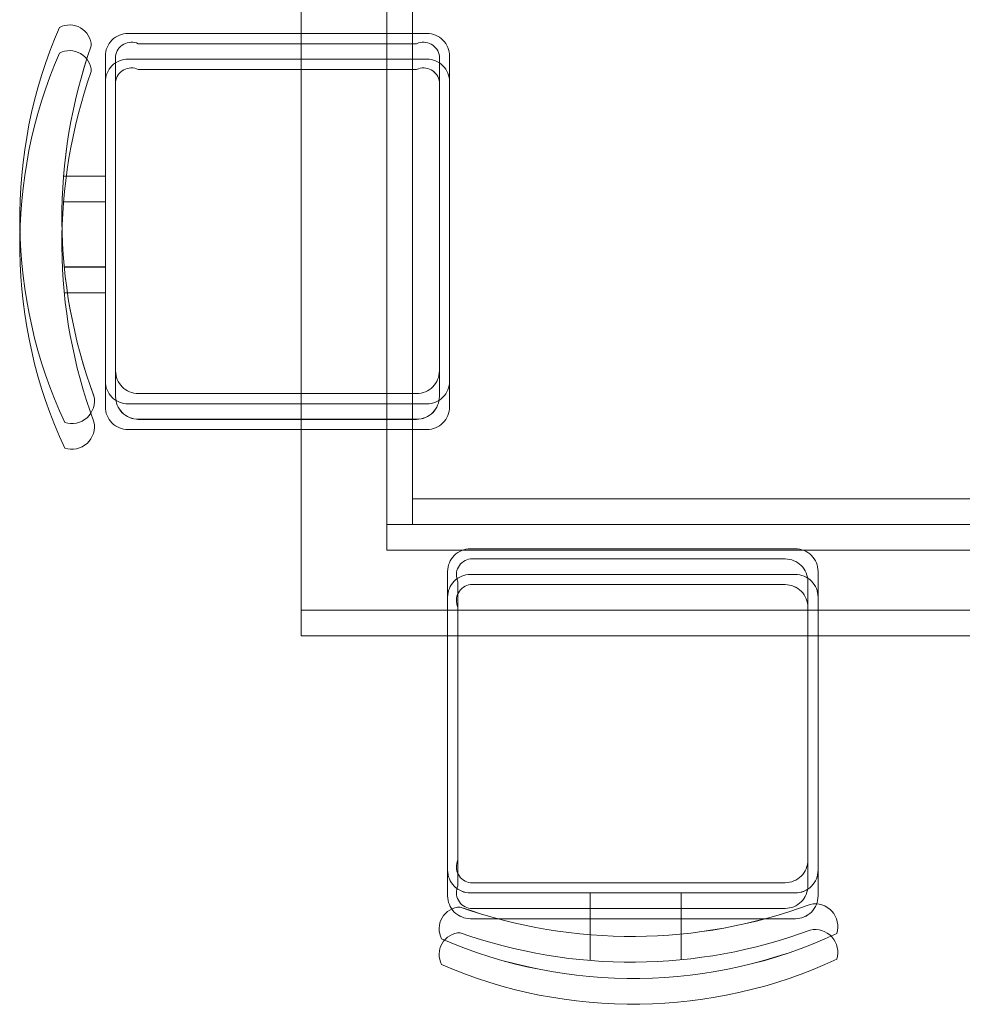
# Model space of a CAD drawing. Units: inches. Extents: x 1885 to 2748, y 783 to 2421.
# Tile 81 of 117: x 2129 to 2156, y 2066 to 2095. Entities that reach past the tile are written whole.
import ezdxf

# ---------------------------------------------------------------- set-up
doc = ezdxf.new("R2010")
doc.units = ezdxf.units.IN
doc.layers.add('A-FURN', color=8, linetype='Continuous', lineweight=13)

# ---------------------------------------------------------------- blocks, each defined once
blk = doc.blocks.new('TABLE-DINING-RECT')
for points in [[(-0.004, 23.421), (37.776, 23.421), (37.776, 0.754), (-0.004, 0.754)], [(-0.004, 23.421), (37.776, 23.421), (37.776, 0.753), (-0.004, 0.753)], [(-0.004, 22.666), (37.776, 22.666), (37.776, -0.002), (-0.004, -0.002)], [(-0.004, 22.665), (37.776, 22.665), (37.776, -0.002), (-0.004, -0.002)], [(2.515, 20.903), (35.257, 20.903), (35.257, 3.272), (2.515, 3.272)], [(2.515, 20.902), (35.257, 20.902), (35.257, 3.272), (2.515, 3.272)], [(2.515, 20.147), (35.257, 20.147), (35.257, 2.517), (2.515, 2.517)], [(2.515, 20.147), (35.257, 20.147), (35.257, 2.516), (2.515, 2.516)], [(3.27, 20.147), (34.501, 20.147), (34.501, 4.028), (3.27, 4.028)], [(3.27, 20.147), (34.501, 20.147), (34.501, 4.027), (3.27, 4.027)], [(3.27, 19.391), (34.501, 19.391), (34.501, 3.272), (3.27, 3.272)], [(3.27, 19.391), (34.501, 19.391), (34.501, 3.272), (3.27, 3.272)]]:
    blk.add_lwpolyline(points, close=True)

msp = doc.modelspace()

# ---------------------------------------------------------------- linework, layer by layer
at = {"layer": 'A-FURN'}
for points in [[(2130.918, 2084.243, -0.578392), (2130.06, 2083.463, -0.214524), (2129.905, 2095.078, -0.552014), (2130.84, 2094.533, 0.175809), (2130.918, 2084.243)], [(2130.918, 2084.242, -0.578392), (2130.06, 2083.463, -0.214524), (2129.905, 2095.078, -0.552014), (2130.84, 2094.532, 0.175809), (2130.918, 2084.242)], [(2131.253, 2094.232, -0.414214), (2131.921, 2094.901), (2140.705, 2094.901, -0.414214), (2141.373, 2094.232), (2141.373, 2084.679, -0.414214), (2140.705, 2084.011), (2131.921, 2084.011, -0.414214), (2131.253, 2084.679), (2131.253, 2094.232)], [(2131.253, 2094.232, -0.414214), (2131.921, 2094.9), (2140.705, 2094.9, -0.414214), (2141.373, 2094.232), (2141.373, 2084.679, -0.414214), (2140.705, 2084.011), (2131.921, 2084.011, -0.414214), (2131.253, 2084.679), (2131.253, 2094.232)], [(2130.918, 2083.487, -0.578392), (2130.06, 2082.708, -0.214524), (2129.905, 2094.323, -0.552014), (2130.84, 2093.777, 0.175809), (2130.918, 2083.487)], [(2130.918, 2083.487, -0.578392), (2130.06, 2082.707, -0.214524), (2129.905, 2094.323, -0.552014), (2130.84, 2093.777, 0.175809), (2130.918, 2083.487)], [(2131.253, 2093.477, -0.414214), (2131.921, 2094.145), (2140.705, 2094.145, -0.414214), (2141.373, 2093.477), (2141.373, 2083.924, -0.414214), (2140.705, 2083.255), (2131.921, 2083.255, -0.414214), (2131.253, 2083.924), (2131.253, 2093.477)], [(2131.253, 2093.476, -0.414214), (2131.921, 2094.145), (2140.705, 2094.145, -0.414214), (2141.373, 2093.476), (2141.373, 2083.923, -0.414214), (2140.705, 2083.255), (2131.921, 2083.255, -0.414214), (2131.253, 2083.923), (2131.253, 2093.476)], [(2131.253, 2088.035), (2130.045, 2088.035, 0.064759)], [(2131.253, 2088.034), (2130.045, 2088.034, 0.064759)], [(2131.253, 2087.279), (2130.045, 2087.279, 0.064759)], [(2131.253, 2087.279), (2130.045, 2087.279, 0.064759)], [(2151.536, 2069.633), (2141.984, 2069.633, -0.414214), (2141.315, 2070.301), (2141.315, 2079.085, -0.414214), (2141.984, 2079.753), (2151.536, 2079.753, -0.414214), (2152.205, 2079.085), (2152.205, 2070.301, -0.414214), (2151.536, 2069.633)], [(2151.536, 2069.632), (2141.984, 2069.632, -0.414214), (2141.315, 2070.301), (2141.315, 2079.085, -0.414214), (2141.984, 2079.753), (2151.536, 2079.753, -0.414214), (2152.205, 2079.085), (2152.205, 2070.301, -0.414214), (2151.536, 2069.632)], [(2151.536, 2068.877), (2141.984, 2068.877, -0.414214), (2141.315, 2069.546), (2141.315, 2078.329, -0.414214), (2141.984, 2078.998), (2151.536, 2078.998, -0.414214), (2152.205, 2078.329), (2152.205, 2069.546, -0.414214), (2151.536, 2068.877)], [(2151.536, 2068.877), (2141.984, 2068.877, -0.414214), (2141.315, 2069.545), (2141.315, 2078.329, -0.414214), (2141.984, 2078.997), (2151.536, 2078.997, -0.414214), (2152.205, 2078.329), (2152.205, 2069.545, -0.414214), (2151.536, 2068.877)], [(2148.181, 2069.633), (2148.181, 2068.425, 0.064759)], [(2148.181, 2069.632), (2148.181, 2068.424, 0.064759)], [(2151.973, 2069.298, -0.578392), (2152.753, 2068.441, -0.214524), (2141.137, 2068.285, -0.552014), (2141.683, 2069.22, 0.175809), (2151.973, 2069.298)], [(2151.973, 2069.297, -0.578392), (2152.753, 2068.44, -0.214524), (2141.137, 2068.284, -0.552014), (2141.683, 2069.219, 0.175809), (2151.973, 2069.297)], [(2148.181, 2068.877), (2148.181, 2067.669, 0.064759)], [(2148.181, 2068.877), (2148.181, 2067.669, 0.064759)], [(2151.973, 2068.542, -0.578392), (2152.753, 2067.685, -0.214524), (2141.137, 2067.529, -0.552014), (2141.683, 2068.464, 0.175809), (2151.973, 2068.542)], [(2151.973, 2068.542, -0.578392), (2152.753, 2067.685, -0.214524), (2141.137, 2067.529, -0.552014), (2141.683, 2068.464, 0.175809), (2151.973, 2068.542)]]:
    msp.add_lwpolyline(points, format="xyb", dxfattribs=at)
for points in [[(2131.554, 2094.228), (2131.554, 2084.98, 0.414214), (2132.222, 2084.312), (2140.404, 2084.312, 0.414214), (2141.072, 2084.98), (2141.072, 2094.228, 0.512069), (2140.404, 2094.599), (2132.222, 2094.599, 0.512069)], [(2131.554, 2094.228), (2131.554, 2084.98, 0.414214), (2132.222, 2084.312), (2140.404, 2084.312, 0.414214), (2141.072, 2084.98), (2141.072, 2094.228, 0.512069), (2140.404, 2094.599), (2132.222, 2094.599, 0.512069)], [(2131.554, 2093.473), (2131.554, 2084.225, 0.414214), (2132.222, 2083.557), (2140.404, 2083.557, 0.414214), (2141.072, 2084.225), (2141.072, 2093.473, 0.512069), (2140.404, 2093.844), (2132.222, 2093.844, 0.512069)], [(2131.554, 2093.472), (2131.554, 2084.224, 0.414214), (2132.222, 2083.556), (2140.404, 2083.556, 0.414214), (2141.072, 2084.224), (2141.072, 2093.472, 0.512069), (2140.404, 2093.844), (2132.222, 2093.844, 0.512069)], [(2141.988, 2069.934), (2151.235, 2069.934, 0.414214), (2151.904, 2070.602), (2151.904, 2078.784, 0.414214), (2151.235, 2079.452), (2141.988, 2079.452, 0.512069), (2141.616, 2078.784), (2141.616, 2070.602, 0.512069)], [(2141.988, 2069.934), (2151.235, 2069.934, 0.414214), (2151.904, 2070.602), (2151.904, 2078.783, 0.414214), (2151.235, 2079.452), (2141.988, 2079.452, 0.512069), (2141.616, 2078.783), (2141.616, 2070.602, 0.512069)], [(2141.988, 2069.178), (2151.235, 2069.178, 0.414214), (2151.904, 2069.847), (2151.904, 2078.028, 0.414214), (2151.235, 2078.697), (2141.988, 2078.697, 0.512069), (2141.616, 2078.028), (2141.616, 2069.847, 0.512069)], [(2141.988, 2069.178), (2151.235, 2069.178, 0.414214), (2151.904, 2069.846), (2151.904, 2078.028, 0.414214), (2151.235, 2078.696), (2141.988, 2078.696, 0.512069), (2141.616, 2078.028), (2141.616, 2069.846, 0.512069)]]:
    msp.add_lwpolyline(points, format="xyb", close=True, dxfattribs=at)
for points in [[(2130.023, 2090.709), (2131.253, 2090.709)], [(2130.023, 2090.708), (2131.253, 2090.708)], [(2130.023, 2089.953), (2131.253, 2089.953)], [(2130.023, 2089.953), (2131.253, 2089.953)], [(2145.507, 2068.403), (2145.507, 2069.633)], [(2145.507, 2068.402), (2145.507, 2069.632)], [(2145.507, 2067.647), (2145.507, 2068.877)], [(2145.507, 2067.647), (2145.507, 2068.877)]]:
    msp.add_lwpolyline(points, dxfattribs=at)

# ---------------------------------------------------------------- block references
msp.add_blockref('TABLE-DINING-RECT', (2137.014, 2077.19), dxfattribs=at)

doc.saveas('drawing.dxf')
